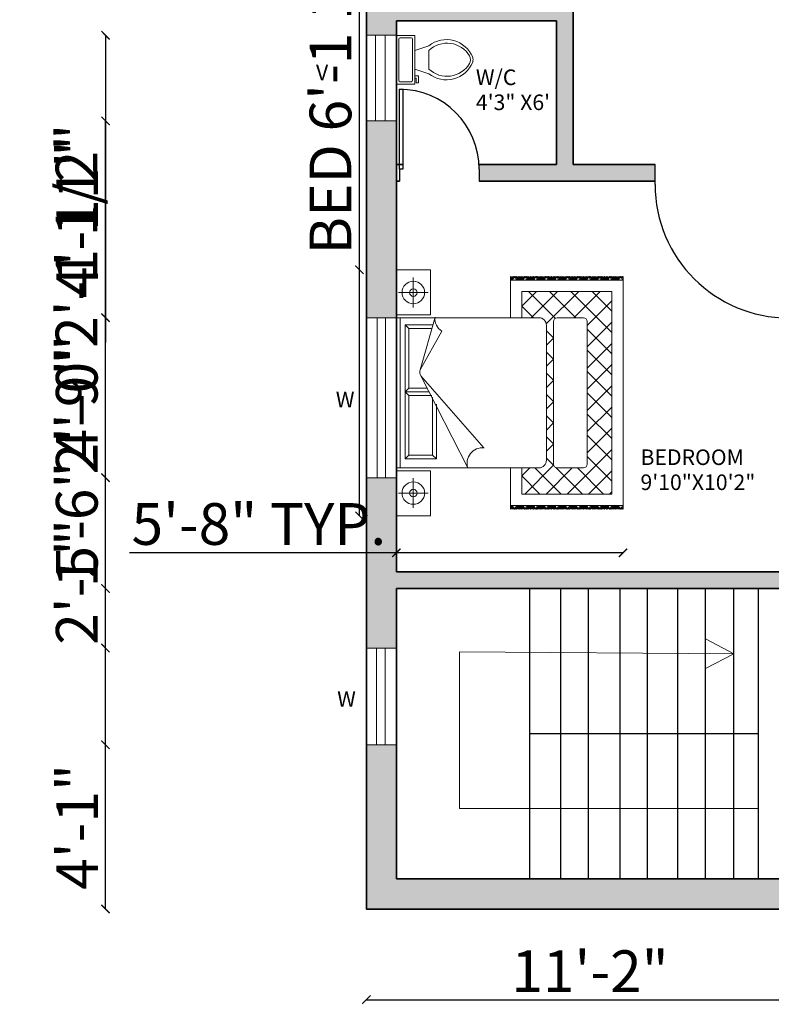
# Model space of a CAD drawing. Units: inches. Extents: x 1750 to 7466, y 1409 to 2004.
# Tile 1 of 5: x 1750 to 1975, y 1420 to 1715. Entities that reach past the tile are written whole.
import ezdxf

# ---------------------------------------------------------------- set-up
doc = ezdxf.new("R2010")
doc.units = ezdxf.units.IN
for name, color, linetype, lineweight in [('A-ANNO-DIMS', 2, 'Continuous', 18), ('A-ANNO-SYMB', 7, 'Continuous', 18), ('A-ANNO-TEXT', 7, 'Continuous', 18), ('A-AREA-IDEN', 7, 'Continuous', 18), ('A-DOOR', 3, 'Continuous', 25), ('A-FLOR-FIXT', 9, 'Continuous', 18), ('A-FLOR-STRS', 7, 'Continuous', 25), ('A-WALL', 7, 'Continuous', 35), ('BEDS', 15, 'Continuous', 18), ('WINDOW', 4, 'Continuous', 18)]:
    doc.layers.add(name, color=color, linetype=linetype, lineweight=lineweight)
doc.layers.add('A-WALL-PATT', color=18, linetype='Continuous', lineweight=13, true_color=0x000000)
doc.styles.get("Standard").update_dxf_attribs({"font": 'arial.ttf'})
doc.dimstyles.new('ISO-25', dxfattribs={"dimtxt": 12.5, "dimasz": 2.5, "dimexe": 1.25, "dimexo": 0.625, "dimtad": 1, "dimdec": 0, "dimlunit": 4, "dimtxsty": 'Standard', "dimblk": 'ARCHTICK', "dimcen": 2.5, "dimse1": 1, "dimse2": 1, "dimclrd": 2, "dimadec": 0, "dimazin": 0, "dimtfac": 1, "dimtdec": 0, "dimtmove": 0, "dimatfit": 3, "dimfxl": 1, "dimarcsym": 0})

# ---------------------------------------------------------------- blocks, each defined once
blk = doc.blocks.new('A$C4CB008C5')
for p, q in [((0, 3.019), (0.6, 3.019)), ((0, 2.569), (0, 3.019)), ((0.6, 3.019), (0.6, 2.569)), ((0.64, 1.121), (0.64, 3.021)), ((0.64, 3.021), (2.64, 3.021)), ((2.64, 3.021), (2.64, 1.121)), ((3.279, 3.019), (2.679, 3.019)), ((2.679, 3.019), (2.679, 2.569)), ((3.279, 2.569), (3.279, 3.019)), ((0.304, 2.6), (0.304, 2.992)), ((0.64, 2.971), (2.64, 2.971)), ((0.759, 2.905), (2.547, 2.905)), ((0.759, 2.489), (0.759, 2.905)), ((0.759, 2.905), (0.809, 2.855)), ((1.603, 2.855), (1.653, 2.905)), ((1.653, 2.905), (1.653, 2.579)), ((1.653, 2.905), (1.703, 2.855)), ((2.497, 2.855), (2.547, 2.905)), ((2.547, 2.905), (2.547, 2.54)), ((2.975, 2.6), (2.975, 2.992)), ((0.106, 2.796), (0.503, 2.796)), ((0.809, 2.855), (1.603, 2.855)), ((0.809, 2.539), (0.809, 2.855)), ((1.603, 2.855), (1.603, 2.551)), ((1.703, 2.855), (1.703, 2.607)), ((1.703, 2.855), (2.497, 2.855)), ((2.497, 2.855), (2.497, 2.556)), ((3.174, 2.796), (2.776, 2.796)), ((0.64, 2.071), (1.866, 2.698)), ((0.906, 1.854), (1.866, 2.698)), ((1.946, 2.705), (2.646, 2.507)), ((1.946, 2.705), (2.46, 2.418)), ((0.6, 2.569), (0, 2.569)), ((0.809, 2.539), (0.759, 2.489)), ((1.58, 2.539), (0.809, 2.539)), ((2.679, 2.569), (3.279, 2.569)), ((1.49, 2.489), (0.759, 2.489)), ((0.907, 1.867), (0.919, 1.867)), ((0.09, 1.5), (0.64, 1.5)), ((0.09, 1.491), (0.099, 1.5)), ((0.09, 1.473), (0.116, 1.5)), ((0.09, 1.456), (0.134, 1.5)), ((0.09, 1.474), (0.09, 1.475)), ((0.09, 1.438), (0.126, 1.474)), ((0.117, 1.43), (0.09, 1.457)), ((0.14, 1.46), (0.108, 1.492)), ((0.14, 1.478), (0.118, 1.5)), ((0.14, 1.496), (0.135, 1.5)), ((0.14, 1.442), (0.135, 1.448)), ((0.14, 0), (0.14, 1.5)), ((2.64, 1.5), (3.19, 1.5)), ((3.14, 1.496), (3.144, 1.5)), ((3.14, 1.478), (3.162, 1.5)), ((3.14, 1.5), (3.14, 0)), ((3.14, 1.46), (3.171, 1.492)), ((3.14, 1.442), (3.145, 1.448)), ((3.19, 1.456), (3.145, 1.5)), ((3.19, 1.438), (3.154, 1.474)), ((3.162, 1.43), (3.19, 1.457)), ((3.19, 1.473), (3.163, 1.5)), ((3.19, 1.491), (3.181, 1.5)), ((3.189, 1.474), (3.19, 1.475)), ((0.14, 1.389), (0.09, 1.439)), ((0.09, 1.42), (0.099, 1.43)), ((0.14, 1.372), (0.09, 1.422)), ((0.09, 1.368), (0.14, 1.417)), ((0.14, 1.354), (0.09, 1.404)), ((0.09, 1.35), (0.14, 1.4)), ((0.14, 1.336), (0.09, 1.386)), ((0.09, 1.332), (0.14, 1.382)), ((0.09, 1.314), (0.14, 1.364)), ((0.09, 1.297), (0.126, 1.333)), ((0.09, 1.333), (0.09, 1.333)), ((0.117, 1.288), (0.09, 1.316)), ((0.14, 1.319), (0.108, 1.35)), ((0.117, 1.412), (0.14, 1.435)), ((0.29, 1.108), (0.532, 1.35)), ((0.29, 0.15), (0.29, 1.35)), ((0.29, 1.35), (0.64, 1.35)), ((0.64, 1.243), (0.533, 1.35)), ((2.64, 1.195), (2.795, 1.35)), ((2.64, 1.35), (2.99, 1.35)), ((2.99, 1.156), (2.795, 1.35)), ((2.99, 1.35), (2.99, 0.15)), ((3.14, 1.389), (3.19, 1.439)), ((3.162, 1.412), (3.14, 1.435)), ((3.14, 1.372), (3.19, 1.422)), ((3.189, 1.368), (3.14, 1.417)), ((3.14, 1.354), (3.19, 1.404)), ((3.19, 1.35), (3.14, 1.4)), ((3.14, 1.336), (3.19, 1.386)), ((3.19, 1.332), (3.14, 1.382)), ((3.19, 1.314), (3.14, 1.364)), ((3.14, 1.319), (3.171, 1.35)), ((3.19, 1.297), (3.154, 1.333)), ((3.162, 1.288), (3.19, 1.316)), ((3.19, 1.42), (3.18, 1.43)), ((3.189, 1.333), (3.19, 1.333)), ((0.14, 1.248), (0.09, 1.298)), ((0.09, 1.279), (0.099, 1.288)), ((0.14, 1.23), (0.09, 1.28)), ((0.09, 1.227), (0.14, 1.276)), ((0.14, 1.213), (0.09, 1.263)), ((0.09, 1.208), (0.14, 1.258)), ((0.14, 1.195), (0.09, 1.245)), ((0.09, 1.19), (0.14, 1.24)), ((0.09, 1.173), (0.14, 1.223)), ((0.09, 1.191), (0.09, 1.192)), ((0.09, 1.155), (0.126, 1.191)), ((0.14, 1.177), (0.108, 1.209)), ((0.117, 1.271), (0.14, 1.294)), ((0.14, 1.301), (0.135, 1.306)), ((0.674, 0.926), (0.29, 1.31)), ((2.632, 0.904), (2.99, 1.262)), ((2.99, 0.873), (2.64, 1.223)), ((3.14, 1.301), (3.145, 1.306)), ((3.14, 1.248), (3.19, 1.298)), ((3.162, 1.271), (3.14, 1.294)), ((3.14, 1.23), (3.19, 1.28)), ((3.189, 1.227), (3.14, 1.276)), ((3.14, 1.213), (3.19, 1.263)), ((3.19, 1.208), (3.14, 1.258)), ((3.14, 1.195), (3.19, 1.245)), ((3.19, 1.19), (3.14, 1.24)), ((3.19, 1.173), (3.14, 1.223)), ((3.14, 1.177), (3.171, 1.209)), ((3.19, 1.155), (3.154, 1.191)), ((3.19, 1.279), (3.18, 1.288)), ((3.189, 1.191), (3.19, 1.192)), ((0.117, 1.147), (0.09, 1.174)), ((0.14, 1.107), (0.09, 1.157)), ((0.09, 1.137), (0.099, 1.147)), ((0.14, 1.089), (0.09, 1.139)), ((0.09, 1.085), (0.14, 1.134)), ((0.14, 1.071), (0.09, 1.121)), ((0.09, 1.067), (0.14, 1.117)), ((0.14, 1.054), (0.09, 1.104)), ((0.09, 1.049), (0.14, 1.099)), ((0.09, 1.031), (0.14, 1.081)), ((0.09, 1.05), (0.09, 1.051)), ((0.09, 1.014), (0.126, 1.05)), ((0.14, 1.036), (0.108, 1.067)), ((0.117, 1.129), (0.14, 1.152)), ((0.14, 1.16), (0.135, 1.165)), ((0.29, 0.825), (0.64, 1.175)), ((3.14, 1.16), (3.145, 1.165)), ((3.14, 1.107), (3.19, 1.157)), ((3.162, 1.129), (3.14, 1.152)), ((3.14, 1.089), (3.19, 1.139)), ((3.189, 1.085), (3.14, 1.134)), ((3.14, 1.071), (3.19, 1.121)), ((3.19, 1.067), (3.14, 1.117)), ((3.14, 1.054), (3.19, 1.104)), ((3.19, 1.049), (3.14, 1.099)), ((3.19, 1.031), (3.14, 1.081)), ((3.14, 1.036), (3.171, 1.067)), ((3.19, 1.014), (3.154, 1.05)), ((3.162, 1.147), (3.19, 1.174)), ((3.19, 1.137), (3.18, 1.147)), ((3.189, 1.05), (3.19, 1.051)), ((0.117, 1.006), (0.09, 1.033)), ((0.14, 0.965), (0.09, 1.015)), ((0.09, 0.996), (0.099, 1.006)), ((0.14, 0.948), (0.09, 0.998)), ((0.09, 0.944), (0.14, 0.993)), ((0.14, 0.93), (0.09, 0.98)), ((0.09, 0.925), (0.14, 0.975)), ((0.14, 0.912), (0.09, 0.962)), ((0.09, 0.908), (0.14, 0.958)), ((0.09, 0.89), (0.14, 0.94)), ((0.14, 0.894), (0.108, 0.926)), ((0.117, 0.988), (0.14, 1.011)), ((0.14, 1.018), (0.135, 1.023)), ((0.64, 0.677), (0.29, 1.027)), ((0.673, 0.925), (0.769, 1.021)), ((0.69, 0.928), (2.59, 0.928)), ((2.54, 1.021), (0.74, 1.021)), ((0.955, 0.928), (0.861, 1.021)), ((0.959, 0.928), (1.052, 1.021)), ((1.238, 0.928), (1.144, 1.021)), ((1.241, 0.928), (1.335, 1.021)), ((1.52, 0.928), (1.427, 1.021)), ((1.524, 0.928), (1.618, 1.021)), ((1.803, 0.928), (1.71, 1.021)), ((1.807, 0.928), (1.9, 1.021)), ((2.086, 0.928), (1.993, 1.021)), ((2.09, 0.928), (2.183, 1.021)), ((2.369, 0.928), (2.276, 1.021)), ((2.373, 0.928), (2.466, 1.021)), ((2.99, 0.59), (2.557, 1.023)), ((2.64, 0.629), (2.99, 0.979)), ((3.14, 1.018), (3.145, 1.023)), ((3.14, 0.965), (3.19, 1.015)), ((3.162, 0.988), (3.14, 1.011)), ((3.14, 0.948), (3.19, 0.998)), ((3.189, 0.944), (3.14, 0.993)), ((3.14, 0.93), (3.19, 0.98)), ((3.19, 0.925), (3.14, 0.975)), ((3.14, 0.912), (3.19, 0.962)), ((3.19, 0.908), (3.14, 0.958)), ((3.19, 0.89), (3.14, 0.94)), ((3.14, 0.894), (3.171, 0.926)), ((3.162, 1.006), (3.19, 1.033)), ((3.19, 0.996), (3.18, 1.006)), ((0.09, 0.908), (0.09, 0.909)), ((0.09, 0.872), (0.126, 0.908)), ((0.117, 0.864), (0.09, 0.891)), ((0.14, 0.824), (0.09, 0.874)), ((0.09, 0.855), (0.099, 0.864)), ((0.14, 0.806), (0.09, 0.856)), ((0.09, 0.802), (0.14, 0.852)), ((0.14, 0.788), (0.09, 0.838)), ((0.09, 0.784), (0.14, 0.834)), ((0.14, 0.771), (0.09, 0.821)), ((0.09, 0.766), (0.14, 0.816)), ((0.09, 0.749), (0.14, 0.799)), ((0.117, 0.847), (0.14, 0.869)), ((0.14, 0.877), (0.135, 0.882)), ((0.29, 0.542), (0.643, 0.895)), ((0.64, 0.878), (0.64, 0.528)), ((2.64, 0.878), (2.64, 0.528)), ((3.14, 0.877), (3.145, 0.882)), ((3.14, 0.824), (3.19, 0.874)), ((3.162, 0.847), (3.14, 0.869)), ((3.14, 0.806), (3.19, 0.856)), ((3.189, 0.802), (3.14, 0.852)), ((3.14, 0.788), (3.19, 0.838)), ((3.19, 0.784), (3.14, 0.834)), ((3.14, 0.771), (3.19, 0.821)), ((3.19, 0.766), (3.14, 0.816)), ((3.19, 0.749), (3.14, 0.799)), ((3.19, 0.872), (3.154, 0.908)), ((3.162, 0.864), (3.19, 0.891)), ((3.19, 0.855), (3.18, 0.864)), ((3.189, 0.908), (3.19, 0.909)), ((0.09, 0.767), (0.09, 0.768)), ((0.09, 0.731), (0.126, 0.767)), ((0.117, 0.723), (0.09, 0.75)), ((0.14, 0.682), (0.09, 0.732)), ((0.09, 0.713), (0.099, 0.723)), ((0.14, 0.665), (0.09, 0.715)), ((0.09, 0.661), (0.14, 0.71)), ((0.14, 0.647), (0.09, 0.697)), ((0.09, 0.642), (0.14, 0.692)), ((0.14, 0.629), (0.09, 0.679)), ((0.09, 0.625), (0.14, 0.675)), ((0.09, 0.607), (0.14, 0.657)), ((0.14, 0.753), (0.108, 0.785)), ((0.117, 0.705), (0.14, 0.728)), ((0.14, 0.735), (0.135, 0.74)), ((0.884, 0.15), (0.29, 0.744)), ((2.443, 0.15), (2.99, 0.696)), ((2.99, 0.307), (2.64, 0.657)), ((3.14, 0.753), (3.171, 0.785)), ((3.14, 0.735), (3.145, 0.74)), ((3.14, 0.682), (3.19, 0.732)), ((3.162, 0.705), (3.14, 0.728)), ((3.14, 0.665), (3.19, 0.715)), ((3.189, 0.661), (3.14, 0.71)), ((3.14, 0.647), (3.19, 0.697)), ((3.19, 0.642), (3.14, 0.692)), ((3.14, 0.629), (3.19, 0.679)), ((3.19, 0.625), (3.14, 0.675)), ((3.19, 0.607), (3.14, 0.657)), ((3.19, 0.731), (3.154, 0.767)), ((3.162, 0.723), (3.19, 0.75)), ((3.19, 0.713), (3.18, 0.723)), ((3.189, 0.767), (3.19, 0.768)), ((0.09, 0.589), (0.126, 0.626)), ((0.09, 0.626), (0.09, 0.626)), ((0.117, 0.581), (0.09, 0.609)), ((0.14, 0.541), (0.09, 0.591)), ((0.09, 0.572), (0.099, 0.581)), ((0.14, 0.523), (0.09, 0.573)), ((0.09, 0.519), (0.14, 0.569)), ((0.14, 0.506), (0.09, 0.556)), ((0.09, 0.501), (0.14, 0.551)), ((0.14, 0.488), (0.09, 0.538)), ((0.09, 0.483), (0.14, 0.533)), ((0.14, 0.612), (0.108, 0.643)), ((0.117, 0.564), (0.14, 0.586)), ((0.14, 0.594), (0.135, 0.599)), ((0.29, 0.259), (0.64, 0.609)), ((3.14, 0.612), (3.171, 0.643)), ((3.14, 0.594), (3.145, 0.599)), ((3.14, 0.541), (3.19, 0.591)), ((3.162, 0.564), (3.14, 0.586)), ((3.14, 0.523), (3.19, 0.573)), ((3.189, 0.519), (3.14, 0.569)), ((3.14, 0.506), (3.19, 0.556)), ((3.19, 0.501), (3.14, 0.551)), ((3.14, 0.488), (3.19, 0.538)), ((3.19, 0.483), (3.14, 0.533)), ((3.19, 0.589), (3.154, 0.626)), ((3.162, 0.581), (3.19, 0.609)), ((3.19, 0.572), (3.18, 0.581)), ((3.189, 0.626), (3.19, 0.626)), ((0.09, 0.466), (0.14, 0.516)), ((0.09, 0.484), (0.09, 0.485)), ((0.09, 0.448), (0.126, 0.484)), ((0.117, 0.44), (0.09, 0.467)), ((0.14, 0.399), (0.09, 0.449)), ((0.09, 0.43), (0.099, 0.44)), ((0.14, 0.382), (0.09, 0.432)), ((0.09, 0.378), (0.14, 0.427)), ((0.14, 0.364), (0.09, 0.414)), ((0.09, 0.36), (0.14, 0.41)), ((0.14, 0.346), (0.09, 0.396)), ((0.14, 0.47), (0.108, 0.502)), ((0.117, 0.422), (0.14, 0.445)), ((0.14, 0.453), (0.135, 0.458)), ((0.601, 0.15), (0.29, 0.462)), ((0.463, 0.15), (0.791, 0.478)), ((0.69, 0.478), (2.59, 0.478)), ((0.746, 0.15), (1.074, 0.478)), ((1.167, 0.15), (0.839, 0.478)), ((1.029, 0.15), (1.357, 0.478)), ((1.45, 0.15), (1.122, 0.478)), ((1.312, 0.15), (1.64, 0.478)), ((1.733, 0.15), (1.405, 0.478)), ((1.595, 0.15), (1.923, 0.478)), ((2.016, 0.15), (1.688, 0.478)), ((1.878, 0.15), (2.206, 0.478)), ((2.298, 0.15), (1.97, 0.478)), ((2.16, 0.15), (2.488, 0.478)), ((2.581, 0.15), (2.253, 0.478)), ((2.864, 0.15), (2.536, 0.478)), ((2.726, 0.15), (2.99, 0.414)), ((3.19, 0.466), (3.14, 0.516)), ((3.14, 0.47), (3.171, 0.502)), ((3.14, 0.453), (3.145, 0.458)), ((3.14, 0.399), (3.19, 0.449)), ((3.162, 0.422), (3.14, 0.445)), ((3.14, 0.382), (3.19, 0.432)), ((3.189, 0.378), (3.14, 0.427)), ((3.14, 0.364), (3.19, 0.414)), ((3.19, 0.36), (3.14, 0.41)), ((3.14, 0.346), (3.19, 0.396)), ((3.19, 0.448), (3.154, 0.484)), ((3.162, 0.44), (3.19, 0.467)), ((3.19, 0.43), (3.18, 0.44)), ((3.189, 0.484), (3.19, 0.485)), ((0.09, 0.342), (0.14, 0.392)), ((0.09, 0.324), (0.14, 0.374)), ((0.09, 0.307), (0.126, 0.343)), ((0.09, 0.343), (0.09, 0.343)), ((0.117, 0.299), (0.09, 0.326)), ((0.14, 0.258), (0.09, 0.308)), ((0.09, 0.289), (0.099, 0.299)), ((0.14, 0.24), (0.09, 0.29)), ((0.09, 0.237), (0.14, 0.286)), ((0.14, 0.223), (0.09, 0.273)), ((0.09, 0.218), (0.14, 0.268)), ((0.14, 0.329), (0.108, 0.36)), ((0.117, 0.281), (0.14, 0.304)), ((0.14, 0.311), (0.135, 0.316)), ((3.19, 0.342), (3.14, 0.392)), ((3.19, 0.324), (3.14, 0.374)), ((3.14, 0.329), (3.171, 0.36)), ((3.14, 0.311), (3.145, 0.316)), ((3.14, 0.258), (3.19, 0.308)), ((3.162, 0.281), (3.14, 0.304)), ((3.14, 0.24), (3.19, 0.29)), ((3.189, 0.237), (3.14, 0.286)), ((3.14, 0.223), (3.19, 0.273)), ((3.19, 0.218), (3.14, 0.268)), ((3.19, 0.307), (3.154, 0.343)), ((3.162, 0.299), (3.19, 0.326)), ((3.19, 0.289), (3.18, 0.299)), ((3.189, 0.343), (3.19, 0.343)), ((0.14, 0.205), (0.09, 0.255)), ((0.09, 0.201), (0.14, 0.251)), ((0.09, 0.183), (0.14, 0.233)), ((0.09, 0.201), (0.09, 0.202)), ((0.09, 0.165), (0.126, 0.201)), ((0.117, 0.157), (0.09, 0.184)), ((0.14, 0.117), (0.09, 0.167)), ((0.09, 0.148), (0.099, 0.157)), ((0.14, 0.099), (0.09, 0.149)), ((0.09, 0.095), (0.14, 0.144)), ((0.14, 0.081), (0.09, 0.131)), ((0.14, 0.187), (0.108, 0.219)), ((0.117, 0.139), (0.14, 0.162)), ((0.14, 0.17), (0.135, 0.175)), ((0.318, 0.15), (0.29, 0.179)), ((2.99, 0.15), (0.29, 0.15)), ((3.14, 0.205), (3.19, 0.255)), ((3.19, 0.201), (3.14, 0.251)), ((3.19, 0.183), (3.14, 0.233)), ((3.14, 0.187), (3.171, 0.219)), ((3.14, 0.17), (3.145, 0.175)), ((3.14, 0.117), (3.19, 0.167)), ((3.162, 0.139), (3.14, 0.162)), ((3.14, 0.099), (3.19, 0.149)), ((3.189, 0.095), (3.14, 0.144)), ((3.14, 0.081), (3.19, 0.131)), ((3.19, 0.165), (3.154, 0.201)), ((3.162, 0.157), (3.19, 0.184)), ((3.19, 0.148), (3.18, 0.157)), ((3.189, 0.201), (3.19, 0.202)), ((0.09, 0.077), (0.14, 0.127)), ((0.14, 0.064), (0.09, 0.114)), ((0.09, 0.059), (0.14, 0.109)), ((0.09, 0.041), (0.14, 0.091)), ((0.09, 0.06), (0.09, 0.061)), ((0.09, 0.024), (0.126, 0.06)), ((0.117, 0.016), (0.09, 0.043)), ((0.115, 0), (0.09, 0.025)), ((0.09, 0.006), (0.099, 0.016)), ((0.097, 0), (0.09, 0.008)), ((0.14, 0.046), (0.108, 0.078)), ((0.119, 0), (0.14, 0.021)), ((0.14, 0.028), (0.135, 0.033)), ((0.137, 0), (0.14, 0.003)), ((3.19, 0.077), (3.14, 0.127)), ((3.14, 0.064), (3.19, 0.114)), ((3.19, 0.059), (3.14, 0.109)), ((3.19, 0.041), (3.14, 0.091)), ((3.14, 0.046), (3.171, 0.078)), ((3.14, 0.028), (3.145, 0.033)), ((3.16, 0), (3.14, 0.021)), ((3.143, 0), (3.14, 0.003)), ((3.19, 0.024), (3.154, 0.06)), ((3.162, 0.016), (3.19, 0.043)), ((3.164, 0), (3.19, 0.025)), ((3.19, 0.006), (3.18, 0.016)), ((3.182, 0), (3.19, 0.008)), ((3.189, 0.06), (3.19, 0.061)), ((0.09, 0), (3.19, 0))]:
    blk.add_line(p, q)
for centre, radius in [((0.304, 2.796), 0.15), ((2.975, 2.796), 0.15), ((0.304, 2.796), 0.05), ((2.975, 2.796), 0.05)]:
    blk.add_circle(centre, radius)
for centre, radius, start, end in [((1.915, 2.61), 0.1, 71.7215, 119.0799), ((2.626, 2.31), 0.198, 84.1725, 146.9889), ((0.7, 1.873), 0.207, 354.6422, 106.9775), ((0.74, 1.121), 0.1, 180, 270), ((2.54, 1.121), 0.1, 270, 0), ((0.69, 0.878), 0.05, 90, 180), ((2.59, 0.878), 0.05, 0, 90), ((0.69, 0.528), 0.05, 180, 270), ((2.59, 0.528), 0.05, 270, 0)]:
    blk.add_arc(centre, radius, start, end)
blk = doc.blocks.new('*U9')
for p, q in [((9.5, -6), (9.5, -2)), ((-8, -8.5), (-8, -8)), ((-7, -8), (-7, -9.5)), ((-4, -8), (-6, -14)), ((4, -8), (6, -14)), ((-10, -8.5), (-8, -8.5)), ((-10, -9.5), (-10, -8.5)), ((-7, -9.5), (-10, -9.5)), ((4, -14), (-4, -14))]:
    blk.add_line(p, q)
blk.add_lwpolyline([(10.5, -8), (10.5, 0), (-10.5, 0), (-10.5, -8)], close=True)
for points in [[(-9.5, -2), (-9.5, -6)], [(8.5, -1), (-8.5, -1)], [(-8.5, -7), (8.5, -7)]]:
    blk.add_lwpolyline(points)
for centre, radius, start, end in [((-8.62, -1.88), 0.884, 81.8699, 188.1301), ((8.62, -1.88), 0.884, 351.8699, 98.1301), ((-8.62, -6.12), 0.884, 171.8699, 278.1301), ((8.62, -6.12), 0.884, 261.8699, 8.1301), ((3.52, -21.58), 12.17, 141.4691, 247.9714), ((4.2, -21.82), 11.33, 136.3677, 238.9468), ((-3.52, -21.58), 12.17, 292.0284, 38.5307), ((-4.2, -21.82), 11.33, 301.053, 43.6321), ((0, -27.88), 4, 245.7318, 294.2682), ((0, -29), 4, 254.8605, 285.1395)]:
    blk.add_arc(centre, radius, start, end)
blk = doc.blocks.new('*U11')
for p, q in [((0, 0), (0, -6)), ((40, 0), (40, -6))]:
    blk.add_line(p, q)
blk.add_lwpolyline([(0, 0), (0, 40), (1.75, 40), (1.75, 0)], close=True)
blk.add_arc((0, 0), 40, 0, 90)
blk = doc.blocks.new('_ArchTick')
at = {"color": 0, "linetype": 'ByBlock', "const_width": 0.15}
blk.add_lwpolyline([(-0.5, -0.5), (0.5, 0.5)], dxfattribs=at)
blk = doc.blocks.new('*D15')
at = {"layer": 'A-ANNO-DIMS', "color": 2, "lineweight": -2, "transparency": 16777216}
for p, q in [((1852.08, 1639.61), (1852.08, 1788.89)), ((1852.08, 1565.91), (1852.08, 1639.61))]:
    blk.add_line(p, q, dxfattribs=at)
at = {"layer": 'Defpoints', "color": 0, "transparency": 16777216}
for p in [(1852.08, 1639.61), (1863.13, 1639.61), (1863.13, 1565.91)]:
    blk.add_point(p, dxfattribs=at)
at = {"layer": 'A-ANNO-DIMS', "color": 2, "lineweight": -2, "transparency": 16777216, "xscale": 2.5, "yscale": 2.5, "zscale": 2.5}
for p, rotation in [((1852.08, 1639.61), 90), ((1852.08, 1565.91), 270)]:
    blk.add_blockref('_ArchTick', p, dxfattribs=dict(at, rotation=rotation))
at = {"layer": 'A-ANNO-DIMS', "color": 0, "transparency": 16777216, "insert": (1844.99, 1715.5), "char_height": 12.5, "attachment_point": 5, "rotation": 90}
blk.add_mtext('BED 6\'-1 1/2" TYP.', dxfattribs=at)
blk = doc.blocks.new('*D16')
at = {"layer": 'A-ANNO-DIMS', "color": 2, "lineweight": -2, "transparency": 16777216}
for p, q in [((1863.13, 1554.85), (1783.19, 1554.85)), ((1931.04, 1554.85), (1863.13, 1554.85))]:
    blk.add_line(p, q, dxfattribs=at)
at = {"layer": 'Defpoints', "color": 0, "transparency": 16777216}
for p in [(1863.13, 1565.91), (1931.04, 1565.91), (1863.13, 1554.85)]:
    blk.add_point(p, dxfattribs=at)
at = {"layer": 'A-ANNO-DIMS', "color": 2, "lineweight": -2, "transparency": 16777216, "xscale": 2.5, "yscale": 2.5, "zscale": 2.5, "rotation": 180}
blk.add_blockref('_ArchTick', (1863.13, 1554.85), dxfattribs=at)
at = {"layer": 'A-ANNO-DIMS', "color": 2, "lineweight": -2, "transparency": 16777216, "xscale": 2.5, "yscale": 2.5, "zscale": 2.5}
blk.add_blockref('_ArchTick', (1931.04, 1554.85), dxfattribs=at)
at = {"layer": 'A-ANNO-DIMS', "color": 0, "transparency": 16777216, "insert": (1821.91, 1561.86), "char_height": 12.5, "attachment_point": 5}
blk.add_mtext('5\'-8" TYP.', dxfattribs=at)
blk = doc.blocks.new('*D26')
at = {"layer": 'A-ANNO-DIMS', "color": 2, "lineweight": -2, "transparency": 16777216}
blk.add_line((1854.13, 1421.02), (1988.13, 1421.02), dxfattribs=at)
at = {"layer": 'Defpoints', "color": 0, "transparency": 16777216}
for p in [(1854.13, 1448.17), (1988.13, 1448.17), (1988.13, 1421.02)]:
    blk.add_point(p, dxfattribs=at)
at = {"layer": 'A-ANNO-DIMS', "color": 2, "lineweight": -2, "transparency": 16777216, "xscale": 2.5, "yscale": 2.5, "zscale": 2.5, "rotation": 180}
blk.add_blockref('_ArchTick', (1854.13, 1421.02), dxfattribs=at)
at = {"layer": 'A-ANNO-DIMS', "color": 2, "lineweight": -2, "transparency": 16777216, "xscale": 2.5, "yscale": 2.5, "zscale": 2.5}
blk.add_blockref('_ArchTick', (1988.13, 1421.02), dxfattribs=at)
at = {"layer": 'A-ANNO-DIMS', "color": 0, "transparency": 16777216, "insert": (1921.13, 1427.92), "char_height": 12.5, "attachment_point": 5}
blk.add_mtext('11\'-2"', dxfattribs=at)
blk = doc.blocks.new('*D27')
at = {"layer": 'A-ANNO-DIMS', "color": 2, "lineweight": -2, "transparency": 16777216}
blk.add_line((1775.98, 1448.17), (1775.98, 1497.36), dxfattribs=at)
at = {"layer": 'Defpoints', "color": 0, "transparency": 16777216}
for p in [(1775.98, 1497.36), (1854.13, 1497.36), (1854.13, 1448.17)]:
    blk.add_point(p, dxfattribs=at)
at = {"layer": 'A-ANNO-DIMS', "color": 2, "lineweight": -2, "transparency": 16777216, "xscale": 2.5, "yscale": 2.5, "zscale": 2.5}
for p, rotation in [((1775.98, 1497.36), 90), ((1775.98, 1448.17), 270)]:
    blk.add_blockref('_ArchTick', p, dxfattribs=dict(at, rotation=rotation))
at = {"layer": 'A-ANNO-DIMS', "color": 0, "transparency": 16777216, "insert": (1769.08, 1472.76), "char_height": 12.5, "attachment_point": 5, "rotation": 90}
blk.add_mtext('4\'-1"', dxfattribs=at)
blk = doc.blocks.new('*D28')
at = {"layer": 'A-ANNO-DIMS', "color": 2, "lineweight": -2, "transparency": 16777216}
for p, q in [((1775.98, 1526.31), (1775.98, 1563.5)), ((1775.98, 1497.36), (1775.98, 1526.31))]:
    blk.add_line(p, q, dxfattribs=at)
at = {"layer": 'Defpoints', "color": 0, "transparency": 16777216}
for p in [(1775.98, 1526.31), (1854.13, 1526.31), (1854.13, 1497.36)]:
    blk.add_point(p, dxfattribs=at)
at = {"layer": 'A-ANNO-DIMS', "color": 2, "lineweight": -2, "transparency": 16777216, "xscale": 2.5, "yscale": 2.5, "zscale": 2.5}
for p, rotation in [((1775.98, 1526.31), 90), ((1775.98, 1497.36), 270)]:
    blk.add_blockref('_ArchTick', p, dxfattribs=dict(at, rotation=rotation))
at = {"layer": 'A-ANNO-DIMS', "color": 0, "transparency": 16777216, "insert": (1768.98, 1546.15), "char_height": 12.5, "attachment_point": 5, "rotation": 90}
blk.add_mtext('2\'-5"', dxfattribs=at)
blk = doc.blocks.new('*D29')
at = {"layer": 'A-ANNO-DIMS', "color": 2, "lineweight": -2, "transparency": 16777216}
for p, q in [((1775.98, 1544.17), (1775.98, 1579.97)), ((1775.98, 1526.31), (1775.98, 1544.17))]:
    blk.add_line(p, q, dxfattribs=at)
at = {"layer": 'Defpoints', "color": 0, "transparency": 16777216}
for p in [(1775.98, 1544.17), (1863.13, 1544.17), (1854.13, 1526.31)]:
    blk.add_point(p, dxfattribs=at)
at = {"layer": 'A-ANNO-DIMS', "color": 2, "lineweight": -2, "transparency": 16777216, "xscale": 2.5, "yscale": 2.5, "zscale": 2.5}
for p, rotation in [((1775.98, 1544.17), 90), ((1775.98, 1526.31), 270)]:
    blk.add_blockref('_ArchTick', p, dxfattribs=dict(at, rotation=rotation))
at = {"layer": 'A-ANNO-DIMS', "color": 0, "transparency": 16777216, "insert": (1768.98, 1563.32), "char_height": 12.5, "attachment_point": 5, "rotation": 90}
blk.add_mtext('1\'-6"', dxfattribs=at)
blk = doc.blocks.new('*D30')
at = {"layer": 'A-ANNO-DIMS', "color": 2, "lineweight": -2, "transparency": 16777216}
for p, q in [((1775.98, 1577.33), (1775.98, 1614.52)), ((1775.98, 1544.17), (1775.98, 1577.33))]:
    blk.add_line(p, q, dxfattribs=at)
at = {"layer": 'Defpoints', "color": 0, "transparency": 16777216}
for p in [(1775.98, 1577.33), (1854.13, 1577.33), (1863.13, 1544.17)]:
    blk.add_point(p, dxfattribs=at)
at = {"layer": 'A-ANNO-DIMS', "color": 2, "lineweight": -2, "transparency": 16777216, "xscale": 2.5, "yscale": 2.5, "zscale": 2.5}
for p, rotation in [((1775.98, 1577.33), 90), ((1775.98, 1544.17), 270)]:
    blk.add_blockref('_ArchTick', p, dxfattribs=dict(at, rotation=rotation))
at = {"layer": 'A-ANNO-DIMS', "color": 0, "transparency": 16777216, "insert": (1768.98, 1597.17), "char_height": 12.5, "attachment_point": 5, "rotation": 90}
blk.add_mtext('2\'-9"', dxfattribs=at)
blk = doc.blocks.new('*D31')
at = {"layer": 'A-ANNO-DIMS', "color": 2, "lineweight": -2, "transparency": 16777216}
blk.add_line((1775.98, 1577.33), (1775.98, 1625.24), dxfattribs=at)
at = {"layer": 'Defpoints', "color": 0, "transparency": 16777216}
for p in [(1775.98, 1625.24), (1854.13, 1625.24), (1854.13, 1577.33)]:
    blk.add_point(p, dxfattribs=at)
at = {"layer": 'A-ANNO-DIMS', "color": 2, "lineweight": -2, "transparency": 16777216, "xscale": 2.5, "yscale": 2.5, "zscale": 2.5}
for p, rotation in [((1775.98, 1625.24), 90), ((1775.98, 1577.33), 270)]:
    blk.add_blockref('_ArchTick', p, dxfattribs=dict(at, rotation=rotation))
at = {"layer": 'A-ANNO-DIMS', "color": 0, "transparency": 16777216, "insert": (1768.98, 1601.28), "char_height": 12.5, "attachment_point": 5, "rotation": 90}
blk.add_mtext('4\'-0"', dxfattribs=at)
blk = doc.blocks.new('*D32')
at = {"layer": 'A-ANNO-DIMS', "color": 2, "lineweight": -2, "transparency": 16777216}
blk.add_line((1775.98, 1625.24), (1775.98, 1684.17), dxfattribs=at)
at = {"layer": 'Defpoints', "color": 0, "transparency": 16777216}
for p in [(1775.98, 1684.17), (1854.13, 1684.17), (1854.13, 1625.24)]:
    blk.add_point(p, dxfattribs=at)
at = {"layer": 'A-ANNO-DIMS', "color": 2, "lineweight": -2, "transparency": 16777216, "xscale": 2.5, "yscale": 2.5, "zscale": 2.5}
for p, rotation in [((1775.98, 1684.17), 90), ((1775.98, 1625.24), 270)]:
    blk.add_blockref('_ArchTick', p, dxfattribs=dict(at, rotation=rotation))
at = {"layer": 'A-ANNO-DIMS', "color": 0, "transparency": 16777216, "insert": (1769.08, 1654.7), "char_height": 12.5, "attachment_point": 5, "rotation": 90}
blk.add_mtext('4\'-11"', dxfattribs=at)
blk = doc.blocks.new('*D33')
at = {"layer": 'A-ANNO-DIMS', "color": 2, "lineweight": -2, "transparency": 16777216}
for p, q in [((1775.98, 1709.82), (1775.98, 1684.17)), ((1775.98, 1684.17), (1775.98, 1617.85))]:
    blk.add_line(p, q, dxfattribs=at)
at = {"layer": 'Defpoints', "color": 0, "transparency": 16777216}
for p in [(1863.13, 1709.82), (1775.98, 1684.17), (1863.13, 1684.17)]:
    blk.add_point(p, dxfattribs=at)
at = {"layer": 'A-ANNO-DIMS', "color": 2, "lineweight": -2, "transparency": 16777216, "xscale": 2.5, "yscale": 2.5, "zscale": 2.5}
for p, rotation in [((1775.98, 1709.82), 90), ((1775.98, 1684.17), 270)]:
    blk.add_blockref('_ArchTick', p, dxfattribs=dict(at, rotation=rotation))
at = {"layer": 'A-ANNO-DIMS', "color": 0, "transparency": 16777216, "insert": (1768.9, 1649.76), "char_height": 12.5, "attachment_point": 5, "rotation": 90}
blk.add_mtext('2\'-1 1/2"', dxfattribs=at)

msp = doc.modelspace()

# ---------------------------------------------------------------- hatches: boundary and pattern name
at = {"layer": 'A-WALL-PATT'}
h = msp.add_hatch(color=256, dxfattribs=at)
h.dxf.hatch_style = 1
h.paths.add_polyline_path([(1896.49, 1928.17), (1854.13, 1928.17), (1854.13, 1893.52), (1863.13, 1893.52), (1863.13, 1919.17), (1896.49, 1919.17)])
h.paths.add_polyline_path([(2022.32, 1928.17), (1945.82, 1928.17), (1945.82, 1919.17), (1983.13, 1919.17), (1983.13, 1804.17), (1974.13, 1804.17), (1974.13, 1799.17), (1995.93, 1799.17), (1995.93, 1804.17), (1988.13, 1804.17), (1988.13, 1919.17), (2022.32, 1919.17)])
h.paths.add_polyline_path([(2094.13, 1928.17), (2070.34, 1928.17), (2070.34, 1919.17), (2085.13, 1919.17), (2085.13, 1875.24), (2094.13, 1875.24)])
h.paths.add_polyline_path([(2094.13, 1827.64), (2085.13, 1827.64), (2085.13, 1804.17), (2035.93, 1804.17), (2035.93, 1799.17), (2085.13, 1799.17), (2085.13, 1763.18), (2094.13, 1763.18)])
h.paths.add_polyline_path([(1863.13, 1846.52), (1854.13, 1846.52), (1854.13, 1751.88), (1863.13, 1751.88)])
h.paths.add_polyline_path([(1934.13, 1804.17), (1863.13, 1804.17), (1863.13, 1799.17), (1911.13, 1799.17), (1911.13, 1794.68), (1912.55, 1794.68), (1916.13, 1794.68), (1916.13, 1799.17), (1934.13, 1799.17)])
h.paths.add_polyline_path([(1863.13, 1726.23), (1854.13, 1726.23), (1854.13, 1709.82), (1863.13, 1709.82), (1863.13, 1714.17), (1911.13, 1714.17), (1911.13, 1671.17), (1887.9, 1671.17, -0.01479), (1887.95, 1669.75), (1887.95, 1666.17), (1916.13, 1666.17), (1940.64, 1666.17), (1940.64, 1671.17), (1916.13, 1671.17), (1916.13, 1770.77), (1912.55, 1770.77, -0.01479), (1911.13, 1770.81), (1911.13, 1719.17), (1863.13, 1719.17)])
h.paths.add_polyline_path([(1863.13, 1684.17), (1854.13, 1684.17), (1854.13, 1625.24), (1863.13, 1625.24)])
h.paths.add_polyline_path([(1863.13, 1577.33), (1854.13, 1577.33), (1854.13, 1526.31), (1863.13, 1526.31), (1863.13, 1544.17), (1983.13, 1544.17), (1988.13, 1544.17), (1990.13, 1544.17), (1990.13, 1549.17), (1990.13, 1620.17), (1996.77, 1620.17), (1996.77, 1625.17), (1990.13, 1625.17), (1990.13, 1666.17), (1990.13, 1671.17), (1980.64, 1671.17), (1980.64, 1666.17), (1985.13, 1666.17), (1985.13, 1625.17), (1985.13, 1549.17), (1863.13, 1549.17)])
h.paths.add_polyline_path([(1988.13, 1457.17), (1863.13, 1457.17), (1863.13, 1497.36), (1854.13, 1497.36), (1854.13, 1448.17), (1988.13, 1448.17)])
h.paths.add_polyline_path([(2031.23, 1454.78), (1988.13, 1454.78), (1988.13, 1450.91), (2031.23, 1450.91)])
h.paths.add_polyline_path([(2074.33, 1454.78), (2037.79, 1454.78), (2037.79, 1450.91), (2074.33, 1450.91)], flags=17)
h.paths.add_polyline_path([(2094.13, 1714.84), (2085.13, 1714.84), (2085.13, 1625.17), (2036.77, 1625.17), (2036.77, 1620.17), (2085.13, 1620.17), (2085.13, 1457.17), (2074.33, 1457.17), (2074.33, 1448.17), (2094.13, 1448.17)])
h.paths.add_polyline_path([(1846.92, 1867), (1855.4, 1867), (1855.4, 1874), (1846.92, 1874)], flags=9)
h.paths.add_polyline_path([(1885.75, 1686.15), (1909.97, 1686.15), (1909.97, 1693.31), (1885.75, 1693.31)], flags=25)
h.paths.add_polyline_path([(1885.73, 1693.64), (1900.82, 1693.64), (1900.82, 1700.88), (1885.73, 1700.88)], flags=25)
h.paths.add_polyline_path([(1866.42, 1762.99), (1892.45, 1762.99), (1892.45, 1770.14), (1866.42, 1770.14)], flags=25)
h.paths.add_polyline_path([(1866.4, 1770.47), (1898.87, 1770.47), (1898.87, 1777.71), (1866.4, 1777.71)], flags=9)
h.paths.add_polyline_path([(1925.02, 1731.07), (1964.24, 1731.07), (1964.24, 1738.22), (1925.02, 1738.22)], flags=9)
h.paths.add_polyline_path([(1925.01, 1738.55), (1982.11, 1738.55), (1982.11, 1745.79), (1925.01, 1745.79)], flags=9)
h.paths.add_polyline_path([(1995.48, 1862.99), (2034.71, 1862.99), (2034.71, 1870.14), (1995.48, 1870.14)], flags=9)
h.paths.add_polyline_path([(1995.47, 1870.47), (2026.49, 1870.47), (2026.49, 1877.71), (1995.47, 1877.71)], flags=9)
h.paths.add_polyline_path([(1869.07, 1829.02), (1905.98, 1829.02), (1905.98, 1836.17), (1869.07, 1836.17)], flags=9)
h.paths.add_polyline_path([(1869.05, 1836.5), (1905.15, 1836.5), (1905.15, 1843.74), (1869.05, 1843.74)], flags=9)

# ---------------------------------------------------------------- linework, layer by layer
at = {"layer": 'A-ANNO-SYMB'}
for p, q in [((1964.24, 1524.58), (1955.69, 1529.08)), ((1955.69, 1529.08), (1955.69, 1520.2)), ((1882.07, 1478.32), (1882.07, 1525.18)), ((1882.07, 1525.18), (1964.24, 1524.58)), ((1955.69, 1520.2), (1964.24, 1524.58)), ((1971.66, 1478.32), (1882.07, 1478.32))]:
    msp.add_line(p, q, dxfattribs=at)
at = {"layer": 'A-FLOR-STRS'}
for p, q in [((1903.1, 1457.17), (1903.1, 1544.17)), ((1912.35, 1457.17), (1912.35, 1544.17)), ((1920.72, 1457.17), (1920.72, 1544.17)), ((1930.2, 1457.17), (1930.2, 1544.17)), ((1938.41, 1457.17), (1938.41, 1544.17)), ((1947.46, 1457.17), (1947.46, 1544.17)), ((1955.69, 1457.17), (1955.69, 1544.17)), ((1964.24, 1457.17), (1964.24, 1544.17)), ((1971.66, 1457.17), (1971.66, 1544.17)), ((1971.66, 1500.67), (1903.1, 1500.67))]:
    msp.add_line(p, q, dxfattribs=at)
at = {"layer": 'A-WALL'}
for p, q in [((1916.13, 1671.17), (1916.13, 1770.77)), ((1863.13, 1714.17), (1911.13, 1714.17)), ((1863.13, 1549.17), (1863.13, 1714.17)), ((1911.13, 1671.17), (1911.13, 1714.17)), ((1863.13, 1671.17), (1865.08, 1671.17)), ((1887.9, 1671.17), (1911.13, 1671.17)), ((1940.64, 1671.17), (1916.13, 1671.17)), ((1863.13, 1666.17), (1864.04, 1666.17)), ((1887.95, 1666.17), (1916.13, 1666.17)), ((1940.64, 1666.17), (1916.13, 1666.17)), ((1863.13, 1549.17), (1985.13, 1549.17)), ((1863.13, 1457.17), (1863.13, 1544.17)), ((1863.13, 1544.17), (1983.13, 1544.17)), ((1988.13, 1457.17), (1863.13, 1457.17))]:
    msp.add_line(p, q, dxfattribs=at)
msp.add_lwpolyline([(1988.13, 1448.17), (1854.13, 1448.17), (1854.13, 1928.17), (2094.13, 1928.17), (2094.13, 1448.17), (2074.33, 1448.17)], dxfattribs=at)
at = {"layer": 'WINDOW'}
for p, q in [((1863.13, 1709.82), (1854.13, 1709.82)), ((1854.13, 1709.82), (1854.13, 1684.17)), ((1856.84, 1709.82), (1856.84, 1684.17)), ((1859.75, 1709.82), (1859.75, 1684.17)), ((1863.13, 1684.17), (1863.13, 1709.82)), ((1854.13, 1684.17), (1863.13, 1684.17)), ((1863.13, 1625.24), (1854.13, 1625.24)), ((1854.13, 1625.24), (1854.13, 1577.33)), ((1857.32, 1625.24), (1857.32, 1577.33)), ((1859.89, 1625.24), (1859.89, 1577.33)), ((1863.19, 1577.33), (1863.13, 1625.24)), ((1854.13, 1577.33), (1863.19, 1577.33)), ((1863.13, 1526.31), (1854.13, 1526.31)), ((1854.13, 1526.31), (1854.13, 1497.36)), ((1857.12, 1526.31), (1857.12, 1497.36)), ((1859.78, 1526.31), (1859.78, 1497.36)), ((1863.13, 1497.36), (1863.13, 1526.31)), ((1854.13, 1497.36), (1863.13, 1497.36))]:
    msp.add_line(p, q, dxfattribs=at)

# ---------------------------------------------------------------- block references
at = {"layer": 'A-DOOR', "xscale": 0.5977371973788693, "yscale": 0.5977371973788693, "zscale": 0.5977371973788693}
msp.add_blockref('*U11', (1864.04, 1669.75), dxfattribs=at)
at = {"layer": 'A-DOOR', "rotation": 180}
msp.add_blockref('*U11', (1980.64, 1665.17), dxfattribs=at)
at = {"layer": 'A-FLOR-FIXT', "xscale": 0.6956310263951816, "yscale": 0.6956310263951816, "zscale": 0.6956310263951816, "rotation": 90}
msp.add_blockref('*U9', (1863.13, 1702.51), dxfattribs=at)
at = {"layer": 'BEDS', "xscale": 22.47616773198522, "yscale": 22.47616773198522, "zscale": 22.47616773198522, "rotation": 90}
msp.add_blockref('A$C4CB008C5', (1931.04, 1565.91), dxfattribs=at)

# ---------------------------------------------------------------- texts
at = {"layer": 'A-ANNO-TEXT'}
for s, p in [('V', (1839.03, 1696.38)), ('W', (1844.98, 1598.39)), ('W', (1845.38, 1508.74))]:
    msp.add_text(s, height=4.67, dxfattribs=at).set_placement(p)
at = {"layer": 'A-AREA-IDEN'}
for s, height, p in [('W/C', 4.666, (1886.94, 1694.92)), ('4\'3" X6\'', 4.666, (1886.94, 1687.43)), ('BEDROOM', 4.666, (1936.26, 1581.14)), ('9\'10"X10\'2"', 4.6662, (1936.26, 1573.64))]:
    msp.add_text(s, height=height, dxfattribs=at).set_placement(p)

# ---------------------------------------------------------------- dimensions: what is measured, and where the dimension line sits
at = {"layer": 'A-ANNO-DIMS'}
for base, p1, p2, angle, text, picture, middle in [((1852.08, 1639.61), (1863.13, 1565.91), (1863.13, 1639.61), 90, 'BED <> TYP.', '*D15', (1844.99, 1715.5)), ((1863.13, 1554.85), (1931.04, 1565.91), (1863.13, 1565.91), 180, '<> TYP.', '*D16', (1821.91, 1561.86))]:
    dim = msp.add_linear_dim(base=base, p1=p1, p2=p2, angle=angle, text=text, dimstyle='ISO-25', override={"dimdec": 1, "dimlfac": 1, "dimrnd": 0, "dimzin": 1, "dimdsep": 46, "dimlunit": 4, "dimfrac": 2}, dxfattribs=at)
    dim.commit()
    dim.dimension.update_dxf_attribs({"geometry": picture, "text_midpoint": middle})
for base, p1, p2, picture, middle in [((1775.9834, 1684.1687), (1863.1334, 1709.8167), (1863.1334, 1684.1687), '*D33', (1768.8952, 1649.7596)), ((1775.98, 1684.17), (1854.13, 1625.24), (1854.13, 1684.17), '*D32', (1769.08, 1654.7)), ((1775.98, 1625.24), (1854.13, 1577.33), (1854.13, 1625.24), '*D31', (1768.98, 1601.28)), ((1775.98, 1577.33), (1863.13, 1544.17), (1854.13, 1577.33), '*D30', (1768.98, 1597.17)), ((1775.98, 1544.17), (1854.13, 1526.31), (1863.13, 1544.17), '*D29', (1768.98, 1563.32)), ((1775.9834, 1526.3082), (1854.1334, 1497.3617), (1854.1334, 1526.3082), '*D28', (1768.9762, 1546.1539)), ((1775.98, 1497.36), (1854.13, 1448.17), (1854.13, 1497.36), '*D27', (1769.08, 1472.76))]:
    dim = msp.add_linear_dim(base=base, p1=p1, p2=p2, angle=90, dimstyle='ISO-25', override={"dimdec": 1, "dimlfac": 1, "dimrnd": 0, "dimzin": 1, "dimdsep": 46, "dimlunit": 4, "dimfrac": 2}, dxfattribs=at)
    dim.commit()
    dim.dimension.update_dxf_attribs({"geometry": picture, "text_midpoint": middle})
dim = msp.add_linear_dim(base=(1988.13, 1421.02), p1=(1854.13, 1448.17), p2=(1988.13, 1448.17), dimstyle='ISO-25', override={"dimdec": 1, "dimlfac": 1, "dimrnd": 0, "dimzin": 1, "dimdsep": 46, "dimlunit": 4, "dimfrac": 2}, dxfattribs=at)
dim.commit()
dim.dimension.update_dxf_attribs({"geometry": '*D26', "text_midpoint": (1921.13, 1427.92)})

doc.saveas('drawing.dxf')
